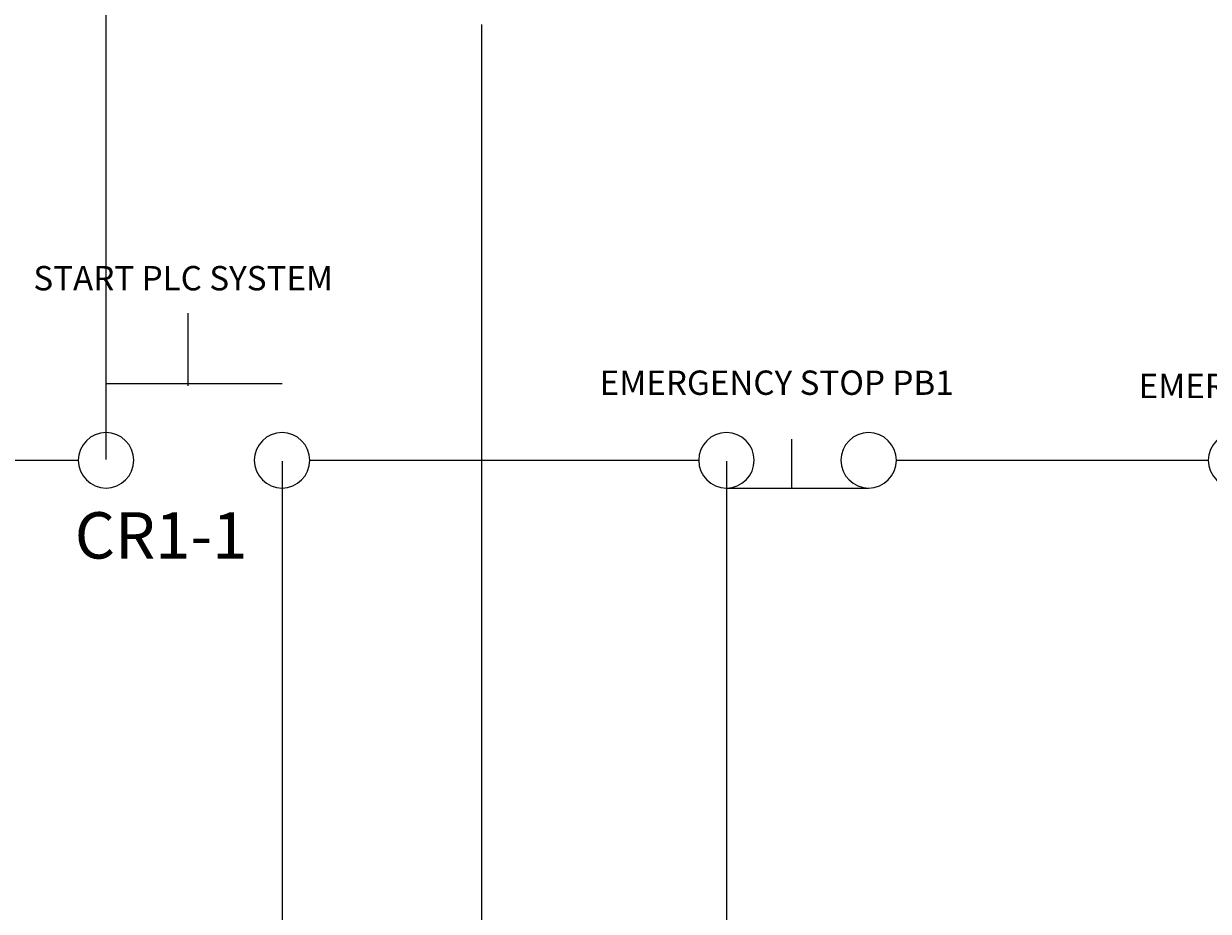
# Model space of a CAD drawing. Units: inches. Extents: x 738 to 1068, y 378 to 757.
# Tile 39 of 41: x 860 to 967, y 606 to 686. Entities that reach past the tile are written whole.
import ezdxf

# ---------------------------------------------------------------- set-up
doc = ezdxf.new("R2010")
doc.units = ezdxf.units.IN
doc.header["$MEASUREMENT"] = 0
for name, color, linetype, lineweight in [('A-ANNO-DIMS', 2, 'Continuous', 18), ('E-ANNO-TEXT', 7, 'Continuous', 18), ('E-CTRL-PBTN', 4, 'Continuous', 25), ('E-CTRL-WIRE', 7, 'Continuous', 18)]:
    doc.layers.add(name, color=color, linetype=linetype, lineweight=lineweight)
doc.styles.get("Standard").update_dxf_attribs({"font": 'arial.ttf'})
doc.dimstyles.get("Standard").update_dxf_attribs({"dimtxt": 0.18, "dimasz": 0.18, "dimexe": 0.18, "dimexo": 0.0625, "dimgap": 0.09, "dimtad": 0, "dimtih": 1, "dimtoh": 1, "dimdec": 4, "dimzin": 0, "dimdsep": 46, "dimtxsty": 'Standard', "dimcen": 0.09, "dimadec": 0, "dimazin": 0, "dimtfac": 1, "dimtdec": 4, "dimtofl": 0, "dimtmove": 0, "dimatfit": 3, "dimfxl": 1, "dimtolj": 1, "dimtzin": 0, "dimarcsym": 0})

# ---------------------------------------------------------------- blocks, each defined once
blk = doc.blocks.new('*D18')
at = {"layer": 'A-ANNO-DIMS', "color": 0, "lineweight": -2, "transparency": 16777216}
for p, q in [((901.52, 738.38), (1068.18, 738.38)), ((1068, 738.2), (1068, 569.17)), ((1068, 399.78), (1068, 568.8)), ((1023.84, 399.6), (1068.18, 399.6))]:
    blk.add_line(p, q, dxfattribs=at)
at = {"layer": 'A-ANNO-DIMS', "color": 0, "transparency": 16777216}
for points in [[(1067.97, 738.2), (1068.03, 738.2), (1068, 738.38)], [(1067.97, 399.78), (1068.03, 399.78), (1068, 399.6)]]:
    blk.add_solid(points, dxfattribs=at)
at = {"layer": 'Defpoints', "color": 0, "transparency": 16777216}
for p in [(901.46, 738.38), (1068, 738.38), (1023.78, 399.6)]:
    blk.add_point(p, dxfattribs=at)
at = {"layer": 'A-ANNO-DIMS', "color": 0, "transparency": 16777216, "insert": (1068, 568.99), "char_height": 0.18, "attachment_point": 5}
blk.add_mtext('\\A1;338.8', dxfattribs=at)
blk = doc.blocks.new('*D26')
at = {"layer": 'A-ANNO-DIMS', "color": 0, "lineweight": -2, "transparency": 16777216}
for p, q in [((816.01, 647.05), (816.01, 756.51)), ((816.19, 756.33), (841.41, 756.33)), ((867.42, 756.33), (842.2, 756.33)), ((867.6, 647.05), (867.6, 756.51))]:
    blk.add_line(p, q, dxfattribs=at)
at = {"layer": 'A-ANNO-DIMS', "color": 0, "transparency": 16777216}
for points in [[(816.19, 756.36), (816.19, 756.3), (816.01, 756.33)], [(867.42, 756.36), (867.42, 756.3), (867.6, 756.33)]]:
    blk.add_solid(points, dxfattribs=at)
at = {"layer": 'Defpoints', "color": 0, "transparency": 16777216}
for p in [(867.6, 756.33), (816.01, 646.99), (867.6, 646.99)]:
    blk.add_point(p, dxfattribs=at)
at = {"layer": 'A-ANNO-DIMS', "color": 0, "transparency": 16777216, "insert": (841.8, 756.33), "char_height": 0.18, "attachment_point": 5}
blk.add_mtext('\\A1;51.59', dxfattribs=at)
blk = doc.blocks.new('*D27')
at = {"layer": 'A-ANNO-DIMS', "color": 0, "lineweight": -2, "transparency": 16777216}
for p, q in [((883.46, 646.92), (883.46, 378.24)), ((923.51, 646.92), (923.51, 378.24)), ((883.64, 378.42), (903.09, 378.42)), ((923.33, 378.42), (903.88, 378.42))]:
    blk.add_line(p, q, dxfattribs=at)
at = {"layer": 'A-ANNO-DIMS', "color": 0, "transparency": 16777216}
for points in [[(883.64, 378.45), (883.64, 378.39), (883.46, 378.42)], [(923.33, 378.45), (923.33, 378.39), (923.51, 378.42)]]:
    blk.add_solid(points, dxfattribs=at)
at = {"layer": 'Defpoints', "color": 0, "transparency": 16777216}
for p in [(883.46, 646.99), (923.51, 646.99), (923.51, 378.42)]:
    blk.add_point(p, dxfattribs=at)
at = {"layer": 'A-ANNO-DIMS', "color": 0, "transparency": 16777216, "insert": (903.48, 378.42), "char_height": 0.18, "attachment_point": 5}
blk.add_mtext('\\A1;40.05', dxfattribs=at)
blk = doc.blocks.new('*D28')
at = {"layer": 'A-ANNO-DIMS', "color": 0, "lineweight": -2, "transparency": 16777216}
for p, q in [((923.51, 646.92), (923.51, 378.24)), ((969.44, 646.92), (969.44, 378.24)), ((923.69, 378.42), (946.08, 378.42)), ((969.26, 378.42), (946.87, 378.42))]:
    blk.add_line(p, q, dxfattribs=at)
at = {"layer": 'A-ANNO-DIMS', "color": 0, "transparency": 16777216}
for points in [[(923.69, 378.45), (923.69, 378.39), (923.51, 378.42)], [(969.26, 378.45), (969.26, 378.39), (969.44, 378.42)]]:
    blk.add_solid(points, dxfattribs=at)
at = {"layer": 'Defpoints', "color": 0, "transparency": 16777216}
for p in [(923.51, 646.99), (969.44, 646.99), (969.44, 378.42)]:
    blk.add_point(p, dxfattribs=at)
at = {"layer": 'A-ANNO-DIMS', "color": 0, "transparency": 16777216, "insert": (946.48, 378.42), "char_height": 0.18, "attachment_point": 5}
blk.add_mtext('\\A1;45.93', dxfattribs=at)
blk = doc.blocks.new('*D35')
at = {"layer": 'A-ANNO-DIMS', "color": 0, "lineweight": -2, "transparency": 16777216}
for p, q in [((855.93, 686.27), (855.93, 378.24)), ((901.43, 686.27), (901.43, 378.24)), ((856.11, 378.42), (878.35, 378.42)), ((901.25, 378.42), (879.01, 378.42))]:
    blk.add_line(p, q, dxfattribs=at)
at = {"layer": 'A-ANNO-DIMS', "color": 0, "transparency": 16777216}
for points in [[(856.11, 378.45), (856.11, 378.39), (855.93, 378.42)], [(901.25, 378.45), (901.25, 378.39), (901.43, 378.42)]]:
    blk.add_solid(points, dxfattribs=at)
at = {"layer": 'Defpoints', "color": 0, "transparency": 16777216}
for p in [(855.93, 686.33), (901.43, 686.33), (901.43, 378.42)]:
    blk.add_point(p, dxfattribs=at)
at = {"layer": 'A-ANNO-DIMS', "color": 0, "transparency": 16777216, "insert": (878.68, 378.42), "char_height": 0.18, "attachment_point": 5}
blk.add_mtext('\\A1;45.5', dxfattribs=at)

msp = doc.modelspace()

# ---------------------------------------------------------------- linework, layer by layer
at = {"layer": 'E-CTRL-PBTN'}
for p, q in [((875.007, 653.7091), (875.007, 660.2523)), ((867.5964, 653.9016), (883.4574, 653.9016)), ((929.3953, 644.4398), (929.3953, 648.8866)), ((923.5105, 644.4853), (936.3276, 644.4853))]:
    msp.add_line(p, q, dxfattribs=at)
for points in [[(865.0964, 646.9853, 1), (870.0964, 646.9853, 1)], [(880.9574, 646.9853, 1), (885.9574, 646.9853, 1)], [(921.0105, 646.9853, 1), (926.0105, 646.9853, 1)], [(933.8276, 646.9853, 1), (938.8276, 646.9853, 1)], [(966.9395, 646.9853, 1), (971.9395, 646.9853, 1)]]:
    msp.add_lwpolyline(points, format="xyb", close=True, dxfattribs=at)
at = {"layer": 'E-CTRL-WIRE'}
for p, q in [((818.5076, 646.9853), (865.0964, 646.9853)), ((885.9574, 646.9853), (921.0105, 646.9853)), ((938.8276, 646.9853), (966.9395, 646.9853))]:
    msp.add_line(p, q, dxfattribs=at)

# ---------------------------------------------------------------- texts
at = {"layer": 'E-ANNO-TEXT'}
for s, height, p in [('START PLC SYSTEM', 2.19392, (861.0446, 662.3002)), ('EMERGENCY STOP PB1', 2.19392, (912.0908, 652.883)), ('EMERGENCY STOP PB2', 2.19392, (960.6679, 652.5875)), ('CR1-1', 4.17507, (864.7774, 638.1322))]:
    msp.add_text(s, height=height, dxfattribs=at).set_placement(p)

# ---------------------------------------------------------------- dimensions: what is measured, and where the dimension line sits
at = {"layer": 'A-ANNO-DIMS'}
for base, p1, p2, override, picture, middle in [((867.5964, 756.3251), (816.0076, 646.9853), (867.5964, 646.9853), {"dimdec": 2, "dimlfac": 1, "dimrnd": 0, "dimzin": 0, "dimdsep": 46, "dimlunit": 2}, '*D26', (841.802, 756.3251)), ((901.4286, 378.4191), (855.9323, 686.329), (901.4286, 686.3292), {"dimdec": 1, "dimlfac": 1, "dimrnd": 0, "dimzin": 0, "dimdsep": 46, "dimlunit": 2}, '*D35', (878.6804, 378.4191)), ((923.5105, 378.4191), (883.4574, 646.9853), (923.5105, 646.9853), {"dimdec": 2, "dimlfac": 1, "dimrnd": 0, "dimzin": 0, "dimdsep": 46, "dimlunit": 2}, '*D27', (903.484, 378.4191)), ((969.4395, 378.4191), (923.5105, 646.9853), (969.4395, 646.9853), {"dimdec": 2, "dimlfac": 1, "dimrnd": 0, "dimzin": 0, "dimdsep": 46, "dimlunit": 2}, '*D28', (946.475, 378.4191))]:
    dim = msp.add_linear_dim(base=base, p1=p1, p2=p2, dimstyle='Standard', override=override, dxfattribs=at)
    dim.commit()
    dim.dimension.update_dxf_attribs({"geometry": picture, "text_midpoint": middle})
dim = msp.add_linear_dim(base=(1067.9992, 738.3751), p1=(1023.779, 399.5952), p2=(901.4622, 738.3751), angle=90, dimstyle='Standard', override={"dimdec": 1, "dimlfac": 1, "dimrnd": 0, "dimzin": 0, "dimdsep": 46, "dimlunit": 2}, dxfattribs=at)
dim.commit()
dim.dimension.update_dxf_attribs({"geometry": '*D18', "text_midpoint": (1067.9992, 568.9851)})

doc.saveas('drawing.dxf')
